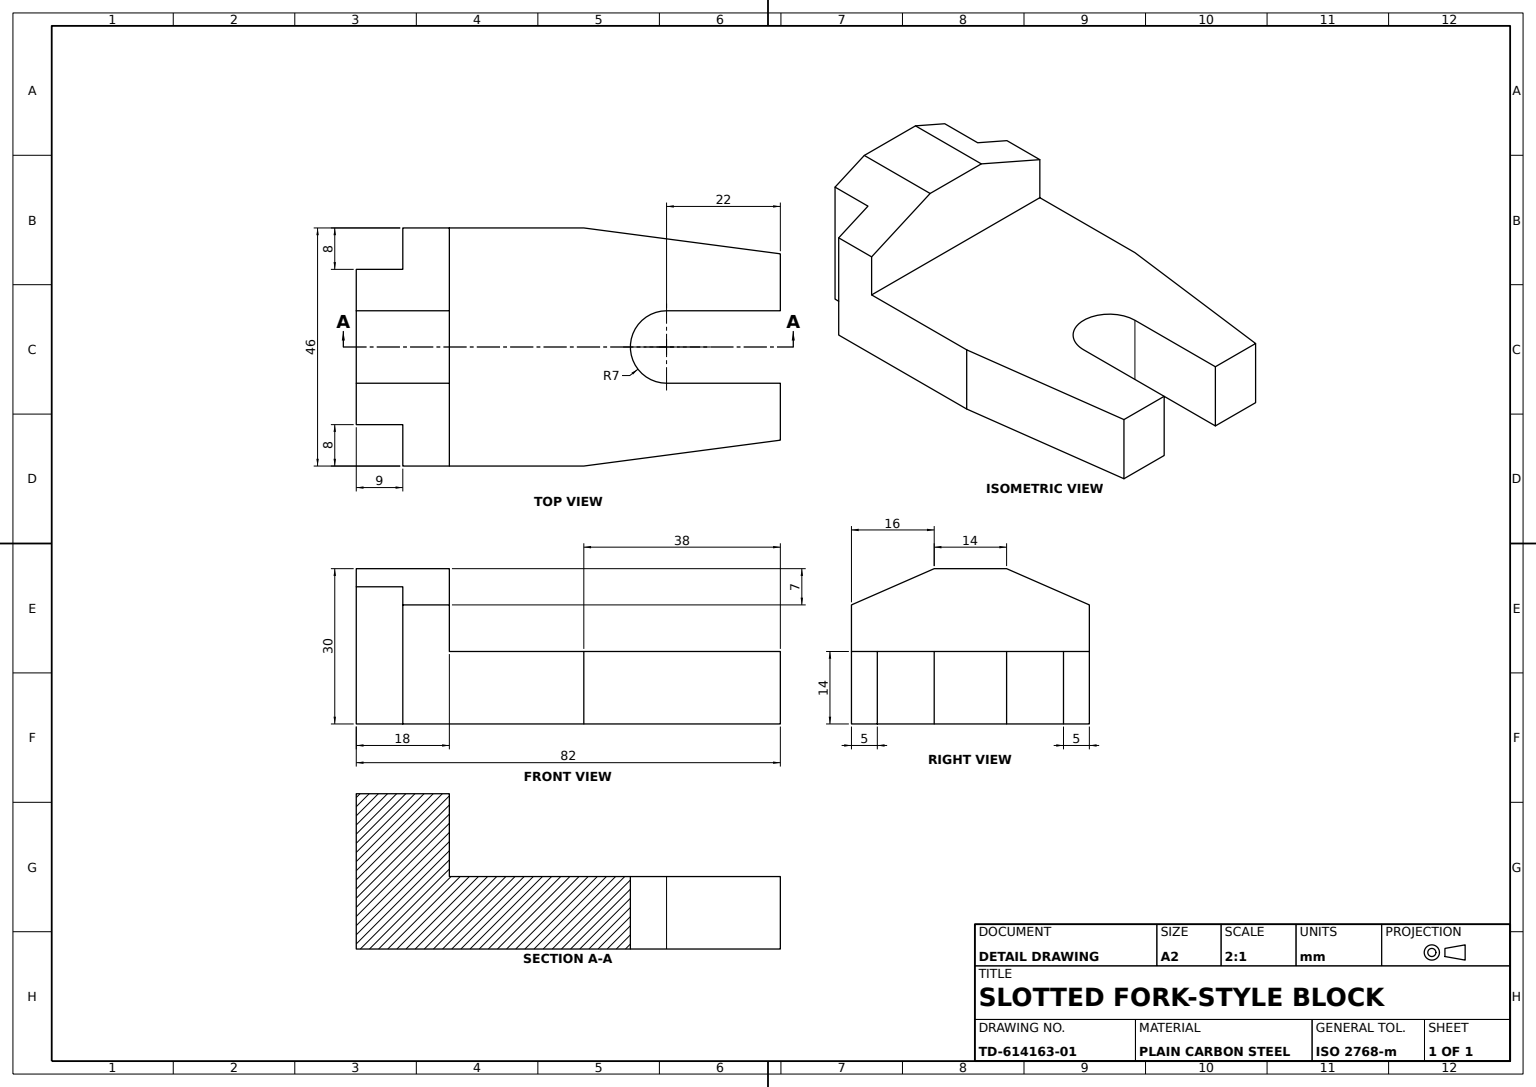
SolidWorks part; units mm, degrees
material "Plain Carbon Steel"
ref_plane "Front Plane" through (0, 0, 0) normal (0, 0, 1) x (1, 0, 0)
ref_plane "Top Plane" through (0, 0, 0) normal (0, 1, 0) x (1, 0, 0)
ref_plane "Right Plane" through (0, 0, 0) normal (1, 0, 0) x (0, 0, -1)
sketch "Base Plate Profile Sketch" plane through (0, 0, 0) normal (0, 1, 0) x (1, 0, 0)
  line L0 (-22, -15) -> (-22, 15)
  line L1 (-13, -23) -> (22, -23)
  line L2 (-22, -15) -> (-22, 15)
  line L3 (-13, 23) -> (22, 23)
  line L4 (22, -23) -> (22, 23)
  line L5 (-14.3478, -15) -> (22, 23) construction
  line L6 (-14.3478, 15) -> (22, -23) construction
  line L7 (-22, 15) -> (-13, 15)
  line L8 (-13, 15) -> (-13, 23)
  line L9 (-22, -15) -> (-13, -15)
  line L10 (-13, -15) -> (-13, -23)
  line L11 (38, 7) -> (60, 7)
  line L12 (60, 18) -> (60, 7)
  line L13 (60, -18) -> (22, -23)
  line L14 (60, 18) -> (22, 23)
  line L16 (60, -7) -> (38, -7)
  line L17 (60, -7) -> (60, -18)
  arc A0 (38, 7) -> (38, -7) centre (38, 0) ccw
  point P0 (0, 0)
  point P9 (-22, 0)
  dimension "D9" = 14
  dimension "D1" = 30
  dimension "D2" = 9
  dimension "D3" = 9
  dimension "D4" = 35
  dimension "D5" = 8
  dimension "D6" = 8
  dimension "D7" = 22
  dimension "D8" = 23
  dimension "D10" = 38
  dimension "D11" = 22
  dimension "D12" = 5
  dimension "D13" = 5
extrude "Slotted Base Plate" add sketch "Base Plate Profile Sketch" along normal blind 14 contours L9 L10 L1 L4 L3 L8 L7 L0 | A0 L11 L12 L14 L4 L13 L17 L16
sketch "Upright Block Sketch" plane through (-22, 0, 0) normal (-1, 0, 0) x (0, 0, 1)
  line L0 (15, 0) -> (-15, 0) construction
  line L1 (7, 30) -> (-7, 30)
  line L4 (-15, 26.5) -> (-7, 30)
  line L5 (7, 30) -> (15, 26.5)
  line L6 (-15, 0) -> (15, 0)
  line L7 (15, 0) -> (15, 26.5)
  line L9 (-15, 26.5) -> (-15, 0)
  dimension "D1" = 14
  dimension "D2" = 7
  dimension "D3" = 30
  dimension "D4" = 26.5
  dimension "D5" = 26.5
  dimension "D6" = 8
  dimension "D7" = 8
extrude "Upright Block" add sketch "Upright Block Sketch" against normal blind 9
sketch "Top Step Sketch" plane through (-13, 0, 0) normal (-1, 0, 0) x (0, 0, 1)
  line L0 (-7, 30) -> (7, 30)
  line L1 (-23, 23) -> (-23, 0)
  line L2 (-23, 0) -> (23, 0)
  line L3 (23, 0) -> (23, 23)
  line L4 (-23, 23) -> (-7, 30)
  line L5 (7, 30) -> (23, 23)
  dimension "D1" = 7
  dimension "D2" = 7
extrude "Top Step Boss" add sketch "Top Step Sketch" against normal blind 9
